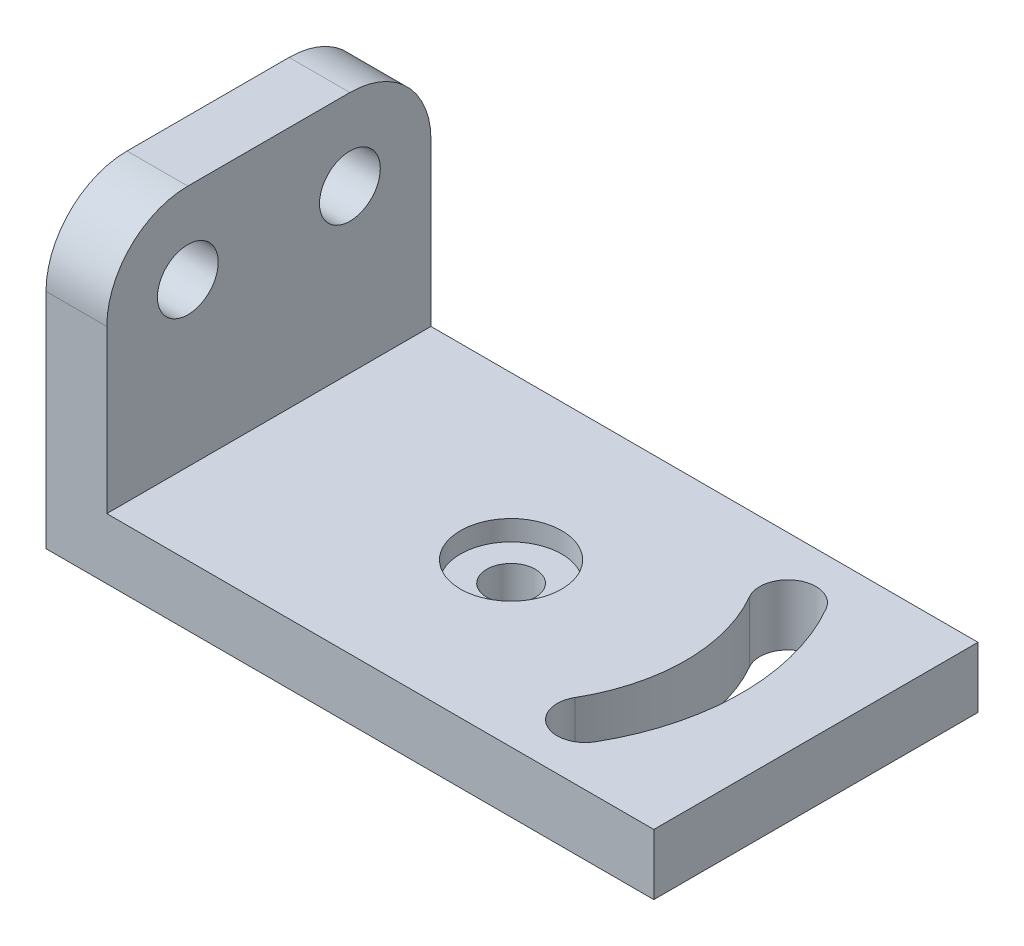
ISO-10303-21;
HEADER;
FILE_DESCRIPTION(('STEP AP214'),'2;1');
FILE_NAME('part.step','',(''),(''),'','','');
FILE_SCHEMA(('AUTOMOTIVE_DESIGN { 1 0 10303 214 1 1 1 1 }'));
ENDSEC;
DATA;
#1=APPLICATION_CONTEXT('core data for automotive mechanical design processes');
#2=APPLICATION_PROTOCOL_DEFINITION('international standard','automotive_design',2000,#1);
#3=PRODUCT_CONTEXT('',#1,'mechanical');
#4=PRODUCT('Part','Part','',(#3));
#5=PRODUCT_RELATED_PRODUCT_CATEGORY('part','',(#4));
#6=PRODUCT_DEFINITION_FORMATION('','',#4);
#7=PRODUCT_DEFINITION_CONTEXT('part definition',#1,'design');
#8=PRODUCT_DEFINITION('design','',#6,#7);
#9=PRODUCT_DEFINITION_SHAPE('','',#8);
#10=(LENGTH_UNIT() NAMED_UNIT(*) SI_UNIT(.MILLI.,.METRE.));
#11=(NAMED_UNIT(*) PLANE_ANGLE_UNIT() SI_UNIT($,.RADIAN.));
#12=(NAMED_UNIT(*) SI_UNIT($,.STERADIAN.) SOLID_ANGLE_UNIT());
#13=UNCERTAINTY_MEASURE_WITH_UNIT(LENGTH_MEASURE(1.E-05),#10,'distance_accuracy_value','');
#14=(GEOMETRIC_REPRESENTATION_CONTEXT(3) GLOBAL_UNCERTAINTY_ASSIGNED_CONTEXT((#13)) GLOBAL_UNIT_ASSIGNED_CONTEXT((#10,
#11,#12)) REPRESENTATION_CONTEXT('',''));
#15=CARTESIAN_POINT('',(0.,0.,0.));
#16=DIRECTION('',(0.,0.,1.));
#17=DIRECTION('',(1.,0.,0.));
#18=AXIS2_PLACEMENT_3D('',#15,#16,#17);
#19=CARTESIAN_POINT('',(0.,15.,40.));
#20=DIRECTION('',(0.,0.,1.));
#21=DIRECTION('',(1.,0.,0.));
#22=AXIS2_PLACEMENT_3D('',#19,#20,#21);
#23=PLANE('',#22);
#24=DIRECTION('',(0.,-1.,0.));
#25=VECTOR('',#24,1.);
#26=CARTESIAN_POINT('',(15.,75.,40.));
#27=LINE('',#26,#25);
#28=CARTESIAN_POINT('',(15.,55.,40.));
#29=VERTEX_POINT('',#28);
#30=CARTESIAN_POINT('',(15.,15.,40.));
#31=VERTEX_POINT('',#30);
#32=EDGE_CURVE('E138',#29,#31,#27,.T.);
#33=ORIENTED_EDGE('',*,*,#32,.F.);
#34=DIRECTION('',(1.,0.,0.));
#35=VECTOR('',#34,1.);
#36=CARTESIAN_POINT('',(0.,55.,40.));
#37=LINE('',#36,#35);
#38=CARTESIAN_POINT('',(0.,55.,40.));
#39=VERTEX_POINT('',#38);
#40=EDGE_CURVE('E11',#29,#39,#37,.F.);
#41=ORIENTED_EDGE('',*,*,#40,.T.);
#42=DIRECTION('',(0.,-1.,0.));
#43=VECTOR('',#42,1.);
#44=CARTESIAN_POINT('',(0.,15.,40.));
#45=LINE('',#44,#43);
#46=CARTESIAN_POINT('',(0.,0.,40.));
#47=VERTEX_POINT('',#46);
#48=EDGE_CURVE('E209',#39,#47,#45,.T.);
#49=ORIENTED_EDGE('',*,*,#48,.T.);
#50=DIRECTION('',(-1.,0.,0.));
#51=VECTOR('',#50,1.);
#52=CARTESIAN_POINT('',(0.,0.,40.));
#53=LINE('',#52,#51);
#54=CARTESIAN_POINT('',(150.,0.,40.));
#55=VERTEX_POINT('',#54);
#56=EDGE_CURVE('E198',#55,#47,#53,.T.);
#57=ORIENTED_EDGE('',*,*,#56,.F.);
#58=DIRECTION('',(0.,-1.,0.));
#59=VECTOR('',#58,1.);
#60=CARTESIAN_POINT('',(150.,15.,40.));
#61=LINE('',#60,#59);
#62=CARTESIAN_POINT('',(150.,15.,40.));
#63=VERTEX_POINT('',#62);
#64=EDGE_CURVE('E216',#63,#55,#61,.T.);
#65=ORIENTED_EDGE('',*,*,#64,.F.);
#66=DIRECTION('',(-1.,0.,0.));
#67=VECTOR('',#66,1.);
#68=CARTESIAN_POINT('',(0.,15.,40.));
#69=LINE('',#68,#67);
#70=EDGE_CURVE('E183',#63,#31,#69,.T.);
#71=ORIENTED_EDGE('',*,*,#70,.T.);
#72=EDGE_LOOP('',(#33,#41,#49,#57,#65,#71));
#73=FACE_BOUND('',#72,.T.);
#74=ADVANCED_FACE('F41',(#73),#23,.T.);
#75=CARTESIAN_POINT('',(150.,15.,0.));
#76=DIRECTION('',(1.,0.,0.));
#77=DIRECTION('',(0.,0.,-1.));
#78=AXIS2_PLACEMENT_3D('',#75,#76,#77);
#79=PLANE('',#78);
#80=DIRECTION('',(0.,0.,1.));
#81=VECTOR('',#80,1.);
#82=CARTESIAN_POINT('',(150.,0.,0.));
#83=LINE('',#82,#81);
#84=CARTESIAN_POINT('',(150.,0.,-40.));
#85=VERTEX_POINT('',#84);
#86=EDGE_CURVE('E203',#85,#55,#83,.T.);
#87=ORIENTED_EDGE('',*,*,#86,.F.);
#88=DIRECTION('',(0.,-1.,0.));
#89=VECTOR('',#88,1.);
#90=CARTESIAN_POINT('',(150.,15.,-40.));
#91=LINE('',#90,#89);
#92=CARTESIAN_POINT('',(150.,15.,-40.));
#93=VERTEX_POINT('',#92);
#94=EDGE_CURVE('E211',#93,#85,#91,.T.);
#95=ORIENTED_EDGE('',*,*,#94,.F.);
#96=DIRECTION('',(0.,0.,1.));
#97=VECTOR('',#96,1.);
#98=CARTESIAN_POINT('',(150.,15.,0.));
#99=LINE('',#98,#97);
#100=EDGE_CURVE('E149',#93,#63,#99,.T.);
#101=ORIENTED_EDGE('',*,*,#100,.T.);
#102=ORIENTED_EDGE('',*,*,#64,.T.);
#103=EDGE_LOOP('',(#87,#95,#101,#102));
#104=FACE_BOUND('',#103,.T.);
#105=ADVANCED_FACE('F283',(#104),#79,.T.);
#106=CARTESIAN_POINT('',(0.,15.,-40.));
#107=DIRECTION('',(0.,0.,-1.));
#108=DIRECTION('',(-1.,0.,0.));
#109=AXIS2_PLACEMENT_3D('',#106,#107,#108);
#110=PLANE('',#109);
#111=DIRECTION('',(0.,-1.,0.));
#112=VECTOR('',#111,1.);
#113=CARTESIAN_POINT('',(0.,15.,-40.));
#114=LINE('',#113,#112);
#115=CARTESIAN_POINT('',(0.,55.,-40.));
#116=VERTEX_POINT('',#115);
#117=CARTESIAN_POINT('',(0.,0.,-40.));
#118=VERTEX_POINT('',#117);
#119=EDGE_CURVE('E212',#116,#118,#114,.T.);
#120=ORIENTED_EDGE('',*,*,#119,.F.);
#121=DIRECTION('',(-1.,0.,0.));
#122=VECTOR('',#121,1.);
#123=CARTESIAN_POINT('',(0.,55.,-40.));
#124=LINE('',#123,#122);
#125=CARTESIAN_POINT('',(15.,55.,-40.));
#126=VERTEX_POINT('',#125);
#127=EDGE_CURVE('E66',#116,#126,#124,.F.);
#128=ORIENTED_EDGE('',*,*,#127,.T.);
#129=DIRECTION('',(0.,-1.,0.));
#130=VECTOR('',#129,1.);
#131=CARTESIAN_POINT('',(15.,75.,-40.));
#132=LINE('',#131,#130);
#133=CARTESIAN_POINT('',(15.,15.,-40.));
#134=VERTEX_POINT('',#133);
#135=EDGE_CURVE('E126',#126,#134,#132,.T.);
#136=ORIENTED_EDGE('',*,*,#135,.T.);
#137=DIRECTION('',(1.,0.,0.));
#138=VECTOR('',#137,1.);
#139=CARTESIAN_POINT('',(0.,15.,-40.));
#140=LINE('',#139,#138);
#141=EDGE_CURVE('E135',#134,#93,#140,.T.);
#142=ORIENTED_EDGE('',*,*,#141,.T.);
#143=ORIENTED_EDGE('',*,*,#94,.T.);
#144=DIRECTION('',(1.,0.,0.));
#145=VECTOR('',#144,1.);
#146=CARTESIAN_POINT('',(0.,0.,-40.));
#147=LINE('',#146,#145);
#148=EDGE_CURVE('E202',#118,#85,#147,.T.);
#149=ORIENTED_EDGE('',*,*,#148,.F.);
#150=EDGE_LOOP('',(#120,#128,#136,#142,#143,#149));
#151=FACE_BOUND('',#150,.T.);
#152=ADVANCED_FACE('F131',(#151),#110,.T.);
#153=CARTESIAN_POINT('',(118.069662559794,15.,-25.0000000000001));
#154=DIRECTION('',(0.,-1.,0.));
#155=DIRECTION('',(0.,0.,-1.));
#156=AXIS2_PLACEMENT_3D('',#153,#154,#155);
#157=CYLINDRICAL_SURFACE('',#156,6.92452153915603);
#158=CARTESIAN_POINT('',(118.069662559794,0.,-25.0000000000001));
#159=DIRECTION('',(0.,1.,0.));
#160=DIRECTION('',(0.,0.,1.));
#161=AXIS2_PLACEMENT_3D('',#158,#159,#160);
#162=CIRCLE('',#161,6.92452153915603);
#163=CARTESIAN_POINT('',(124.066474121756,0.,-28.4622607695782));
#164=VERTEX_POINT('',#163);
#165=CARTESIAN_POINT('',(112.072850997832,0.,-21.5377392304221));
#166=VERTEX_POINT('',#165);
#167=EDGE_CURVE('E168',#164,#166,#162,.T.);
#168=ORIENTED_EDGE('',*,*,#167,.F.);
#169=DIRECTION('',(0.,-1.,0.));
#170=VECTOR('',#169,1.);
#171=CARTESIAN_POINT('',(124.066474121756,15.,-28.4622607695782));
#172=LINE('',#171,#170);
#173=CARTESIAN_POINT('',(124.066474121756,15.,-28.4622607695782));
#174=VERTEX_POINT('',#173);
#175=EDGE_CURVE('E215',#174,#164,#172,.T.);
#176=ORIENTED_EDGE('',*,*,#175,.F.);
#177=CARTESIAN_POINT('',(118.069662559794,15.,-25.0000000000001));
#178=DIRECTION('',(0.,1.,0.));
#179=DIRECTION('',(0.,0.,1.));
#180=AXIS2_PLACEMENT_3D('',#177,#178,#179);
#181=CIRCLE('',#180,6.92452153915603);
#182=CARTESIAN_POINT('',(112.072850997832,15.,-21.5377392304221));
#183=VERTEX_POINT('',#182);
#184=EDGE_CURVE('E169',#174,#183,#181,.T.);
#185=ORIENTED_EDGE('',*,*,#184,.T.);
#186=DIRECTION('',(0.,-1.,0.));
#187=VECTOR('',#186,1.);
#188=CARTESIAN_POINT('',(112.072850997832,15.,-21.5377392304221));
#189=LINE('',#188,#187);
#190=EDGE_CURVE('E146',#183,#166,#189,.T.);
#191=ORIENTED_EDGE('',*,*,#190,.T.);
#192=EDGE_LOOP('',(#168,#176,#185,#191));
#193=FACE_BOUND('',#192,.T.);
#194=ADVANCED_FACE('F317',(#193),#157,.F.);
#195=CARTESIAN_POINT('',(74.7683923705722,15.,0.));
#196=DIRECTION('',(0.,-1.,0.));
#197=DIRECTION('',(0.,0.,-1.));
#198=AXIS2_PLACEMENT_3D('',#195,#196,#197);
#199=CYLINDRICAL_SURFACE('',#198,56.924521539156);
#200=CARTESIAN_POINT('',(74.7683923705722,0.,0.));
#201=DIRECTION('',(0.,1.,0.));
#202=DIRECTION('',(0.,0.,1.));
#203=AXIS2_PLACEMENT_3D('',#200,#201,#202);
#204=CIRCLE('',#203,56.924521539156);
#205=CARTESIAN_POINT('',(124.066474121756,0.,28.4622607695781));
#206=VERTEX_POINT('',#205);
#207=EDGE_CURVE('E186',#206,#164,#204,.T.);
#208=ORIENTED_EDGE('',*,*,#207,.F.);
#209=DIRECTION('',(0.,-1.,0.));
#210=VECTOR('',#209,1.);
#211=CARTESIAN_POINT('',(124.066474121756,15.,28.4622607695781));
#212=LINE('',#211,#210);
#213=CARTESIAN_POINT('',(124.066474121756,15.,28.4622607695781));
#214=VERTEX_POINT('',#213);
#215=EDGE_CURVE('E225',#214,#206,#212,.T.);
#216=ORIENTED_EDGE('',*,*,#215,.F.);
#217=CARTESIAN_POINT('',(74.7683923705722,15.,0.));
#218=DIRECTION('',(0.,1.,0.));
#219=DIRECTION('',(0.,0.,1.));
#220=AXIS2_PLACEMENT_3D('',#217,#218,#219);
#221=CIRCLE('',#220,56.924521539156);
#222=EDGE_CURVE('E175',#214,#174,#221,.T.);
#223=ORIENTED_EDGE('',*,*,#222,.T.);
#224=ORIENTED_EDGE('',*,*,#175,.T.);
#225=EDGE_LOOP('',(#208,#216,#223,#224));
#226=FACE_BOUND('',#225,.T.);
#227=ADVANCED_FACE('F312',(#226),#199,.F.);
#228=CARTESIAN_POINT('',(118.069662559794,15.,25.0000000000001));
#229=DIRECTION('',(0.,-1.,0.));
#230=DIRECTION('',(0.,0.,-1.));
#231=AXIS2_PLACEMENT_3D('',#228,#229,#230);
#232=CYLINDRICAL_SURFACE('',#231,6.92452153915602);
#233=CARTESIAN_POINT('',(118.069662559794,0.,25.0000000000001));
#234=DIRECTION('',(0.,1.,0.));
#235=DIRECTION('',(0.,0.,1.));
#236=AXIS2_PLACEMENT_3D('',#233,#234,#235);
#237=CIRCLE('',#236,6.92452153915602);
#238=CARTESIAN_POINT('',(112.072850997833,0.,21.537739230422));
#239=VERTEX_POINT('',#238);
#240=EDGE_CURVE('E195',#239,#206,#237,.T.);
#241=ORIENTED_EDGE('',*,*,#240,.F.);
#242=DIRECTION('',(0.,-1.,0.));
#243=VECTOR('',#242,1.);
#244=CARTESIAN_POINT('',(112.072850997833,15.,21.537739230422));
#245=LINE('',#244,#243);
#246=CARTESIAN_POINT('',(112.072850997833,15.,21.537739230422));
#247=VERTEX_POINT('',#246);
#248=EDGE_CURVE('E219',#247,#239,#245,.T.);
#249=ORIENTED_EDGE('',*,*,#248,.F.);
#250=CARTESIAN_POINT('',(118.069662559794,15.,25.0000000000001));
#251=DIRECTION('',(0.,1.,0.));
#252=DIRECTION('',(0.,0.,1.));
#253=AXIS2_PLACEMENT_3D('',#250,#251,#252);
#254=CIRCLE('',#253,6.92452153915602);
#255=EDGE_CURVE('E176',#247,#214,#254,.T.);
#256=ORIENTED_EDGE('',*,*,#255,.T.);
#257=ORIENTED_EDGE('',*,*,#215,.T.);
#258=EDGE_LOOP('',(#241,#249,#256,#257));
#259=FACE_BOUND('',#258,.T.);
#260=ADVANCED_FACE('F306',(#259),#232,.F.);
#261=CARTESIAN_POINT('',(74.7683923705722,15.,0.));
#262=DIRECTION('',(0.,-1.,0.));
#263=DIRECTION('',(0.,0.,-1.));
#264=AXIS2_PLACEMENT_3D('',#261,#262,#263);
#265=CYLINDRICAL_SURFACE('',#264,12.5);
#266=CARTESIAN_POINT('',(74.7683923705722,10.,0.));
#267=DIRECTION('',(0.,1.,0.));
#268=DIRECTION('',(0.,0.,1.));
#269=AXIS2_PLACEMENT_3D('',#266,#267,#268);
#270=CIRCLE('',#269,12.5);
#271=CARTESIAN_POINT('',(74.7683923705722,10.,12.5));
#272=VERTEX_POINT('',#271);
#273=EDGE_CURVE('E218',#272,#272,#270,.T.);
#274=ORIENTED_EDGE('',*,*,#273,.F.);
#275=EDGE_LOOP('',(#274));
#276=FACE_BOUND('',#275,.T.);
#277=CARTESIAN_POINT('',(74.7683923705722,15.,0.));
#278=DIRECTION('',(0.,1.,0.));
#279=DIRECTION('',(0.,0.,1.));
#280=AXIS2_PLACEMENT_3D('',#277,#278,#279);
#281=CIRCLE('',#280,12.5);
#282=CARTESIAN_POINT('',(74.7683923705722,15.,12.5));
#283=VERTEX_POINT('',#282);
#284=EDGE_CURVE('E181',#283,#283,#281,.T.);
#285=ORIENTED_EDGE('',*,*,#284,.T.);
#286=EDGE_LOOP('',(#285));
#287=FACE_BOUND('',#286,.T.);
#288=ADVANCED_FACE('F303',(#276,#287),#265,.F.);
#289=CARTESIAN_POINT('',(74.7683923705722,15.,0.));
#290=DIRECTION('',(0.,-1.,0.));
#291=DIRECTION('',(0.,0.,-1.));
#292=AXIS2_PLACEMENT_3D('',#289,#290,#291);
#293=CYLINDRICAL_SURFACE('',#292,43.075478460844);
#294=CARTESIAN_POINT('',(74.7683923705722,0.,0.));
#295=DIRECTION('',(0.,1.,0.));
#296=DIRECTION('',(0.,0.,1.));
#297=AXIS2_PLACEMENT_3D('',#294,#295,#296);
#298=CIRCLE('',#297,43.075478460844);
#299=EDGE_CURVE('E193',#239,#166,#298,.T.);
#300=ORIENTED_EDGE('',*,*,#299,.T.);
#301=ORIENTED_EDGE('',*,*,#190,.F.);
#302=CARTESIAN_POINT('',(74.7683923705722,15.,0.));
#303=DIRECTION('',(0.,1.,0.));
#304=DIRECTION('',(0.,0.,1.));
#305=AXIS2_PLACEMENT_3D('',#302,#303,#304);
#306=CIRCLE('',#305,43.075478460844);
#307=EDGE_CURVE('E177',#247,#183,#306,.T.);
#308=ORIENTED_EDGE('',*,*,#307,.F.);
#309=ORIENTED_EDGE('',*,*,#248,.T.);
#310=EDGE_LOOP('',(#300,#301,#308,#309));
#311=FACE_BOUND('',#310,.T.);
#312=ADVANCED_FACE('F261',(#311),#293,.T.);
#313=CARTESIAN_POINT('',(0.,15.,0.));
#314=DIRECTION('',(1.,0.,0.));
#315=DIRECTION('',(0.,0.,-1.));
#316=AXIS2_PLACEMENT_3D('',#313,#314,#315);
#317=PLANE('',#316);
#318=CARTESIAN_POINT('',(0.,55.,-20.));
#319=DIRECTION('',(1.,0.,0.));
#320=DIRECTION('',(0.,0.,-1.));
#321=AXIS2_PLACEMENT_3D('',#318,#319,#320);
#322=CIRCLE('',#321,7.5);
#323=CARTESIAN_POINT('',(0.,55.,-27.5));
#324=VERTEX_POINT('',#323);
#325=EDGE_CURVE('E153',#324,#324,#322,.T.);
#326=ORIENTED_EDGE('',*,*,#325,.T.);
#327=EDGE_LOOP('',(#326));
#328=FACE_BOUND('',#327,.T.);
#329=CARTESIAN_POINT('',(0.,55.,20.));
#330=DIRECTION('',(1.,0.,0.));
#331=DIRECTION('',(0.,0.,-1.));
#332=AXIS2_PLACEMENT_3D('',#329,#330,#331);
#333=CIRCLE('',#332,7.5);
#334=CARTESIAN_POINT('',(0.,55.,12.5));
#335=VERTEX_POINT('',#334);
#336=EDGE_CURVE('E241',#335,#335,#333,.T.);
#337=ORIENTED_EDGE('',*,*,#336,.T.);
#338=EDGE_LOOP('',(#337));
#339=FACE_BOUND('',#338,.T.);
#340=DIRECTION('',(0.,0.,1.));
#341=VECTOR('',#340,1.);
#342=CARTESIAN_POINT('',(0.,75.,-40.));
#343=LINE('',#342,#341);
#344=CARTESIAN_POINT('',(0.,75.,-20.));
#345=VERTEX_POINT('',#344);
#346=CARTESIAN_POINT('',(0.,75.,20.));
#347=VERTEX_POINT('',#346);
#348=EDGE_CURVE('E155',#345,#347,#343,.T.);
#349=ORIENTED_EDGE('',*,*,#348,.F.);
#350=CARTESIAN_POINT('',(0.,55.,-20.));
#351=DIRECTION('',(1.,0.,0.));
#352=DIRECTION('',(0.,0.,-1.));
#353=AXIS2_PLACEMENT_3D('',#350,#351,#352);
#354=CIRCLE('',#353,20.);
#355=EDGE_CURVE('E232',#345,#116,#354,.F.);
#356=ORIENTED_EDGE('',*,*,#355,.T.);
#357=ORIENTED_EDGE('',*,*,#119,.T.);
#358=DIRECTION('',(0.,0.,1.));
#359=VECTOR('',#358,1.);
#360=CARTESIAN_POINT('',(0.,0.,0.));
#361=LINE('',#360,#359);
#362=EDGE_CURVE('E173',#118,#47,#361,.T.);
#363=ORIENTED_EDGE('',*,*,#362,.T.);
#364=ORIENTED_EDGE('',*,*,#48,.F.);
#365=CARTESIAN_POINT('',(0.,55.,20.));
#366=DIRECTION('',(1.,0.,0.));
#367=DIRECTION('',(0.,0.,-1.));
#368=AXIS2_PLACEMENT_3D('',#365,#366,#367);
#369=CIRCLE('',#368,20.);
#370=EDGE_CURVE('E231',#39,#347,#369,.F.);
#371=ORIENTED_EDGE('',*,*,#370,.T.);
#372=EDGE_LOOP('',(#349,#356,#357,#363,#364,#371));
#373=FACE_BOUND('',#372,.T.);
#374=ADVANCED_FACE('F256',(#328,#339,#373),#317,.F.);
#375=CARTESIAN_POINT('',(0.,15.,0.));
#376=DIRECTION('',(0.,1.,0.));
#377=DIRECTION('',(0.,0.,1.));
#378=AXIS2_PLACEMENT_3D('',#375,#376,#377);
#379=PLANE('',#378);
#380=DIRECTION('',(0.,0.,-1.));
#381=VECTOR('',#380,1.);
#382=CARTESIAN_POINT('',(15.,15.,-40.));
#383=LINE('',#382,#381);
#384=EDGE_CURVE('E143',#31,#134,#383,.T.);
#385=ORIENTED_EDGE('',*,*,#384,.F.);
#386=ORIENTED_EDGE('',*,*,#70,.F.);
#387=ORIENTED_EDGE('',*,*,#100,.F.);
#388=ORIENTED_EDGE('',*,*,#141,.F.);
#389=EDGE_LOOP('',(#385,#386,#387,#388));
#390=FACE_BOUND('',#389,.T.);
#391=ORIENTED_EDGE('',*,*,#184,.F.);
#392=ORIENTED_EDGE('',*,*,#222,.F.);
#393=ORIENTED_EDGE('',*,*,#255,.F.);
#394=ORIENTED_EDGE('',*,*,#307,.T.);
#395=EDGE_LOOP('',(#391,#392,#393,#394));
#396=FACE_BOUND('',#395,.T.);
#397=ORIENTED_EDGE('',*,*,#284,.F.);
#398=EDGE_LOOP('',(#397));
#399=FACE_BOUND('',#398,.T.);
#400=ADVANCED_FACE('F145',(#390,#396,#399),#379,.T.);
#401=CARTESIAN_POINT('',(0.,0.,0.));
#402=DIRECTION('',(0.,1.,0.));
#403=DIRECTION('',(0.,0.,1.));
#404=AXIS2_PLACEMENT_3D('',#401,#402,#403);
#405=PLANE('',#404);
#406=ORIENTED_EDGE('',*,*,#167,.T.);
#407=ORIENTED_EDGE('',*,*,#299,.F.);
#408=ORIENTED_EDGE('',*,*,#240,.T.);
#409=ORIENTED_EDGE('',*,*,#207,.T.);
#410=EDGE_LOOP('',(#406,#407,#408,#409));
#411=FACE_BOUND('',#410,.T.);
#412=ORIENTED_EDGE('',*,*,#56,.T.);
#413=ORIENTED_EDGE('',*,*,#362,.F.);
#414=ORIENTED_EDGE('',*,*,#148,.T.);
#415=ORIENTED_EDGE('',*,*,#86,.T.);
#416=EDGE_LOOP('',(#412,#413,#414,#415));
#417=FACE_BOUND('',#416,.T.);
#418=CARTESIAN_POINT('',(74.7683923705722,0.,0.));
#419=DIRECTION('',(0.,1.,0.));
#420=DIRECTION('',(0.,0.,1.));
#421=AXIS2_PLACEMENT_3D('',#418,#419,#420);
#422=CIRCLE('',#421,6.00000000000001);
#423=CARTESIAN_POINT('',(74.7683923705722,0.,6.00000000000001));
#424=VERTEX_POINT('',#423);
#425=EDGE_CURVE('E162',#424,#424,#422,.T.);
#426=ORIENTED_EDGE('',*,*,#425,.T.);
#427=EDGE_LOOP('',(#426));
#428=FACE_BOUND('',#427,.T.);
#429=ADVANCED_FACE('F276',(#411,#417,#428),#405,.F.);
#430=CARTESIAN_POINT('',(74.7683923705722,10.,0.));
#431=DIRECTION('',(0.,-1.,0.));
#432=DIRECTION('',(0.,0.,-1.));
#433=AXIS2_PLACEMENT_3D('',#430,#431,#432);
#434=CYLINDRICAL_SURFACE('',#433,6.00000000000001);
#435=CARTESIAN_POINT('',(74.7683923705722,10.,0.));
#436=DIRECTION('',(0.,1.,0.));
#437=DIRECTION('',(0.,0.,1.));
#438=AXIS2_PLACEMENT_3D('',#435,#436,#437);
#439=CIRCLE('',#438,6.00000000000001);
#440=CARTESIAN_POINT('',(74.7683923705722,10.,6.00000000000001));
#441=VERTEX_POINT('',#440);
#442=EDGE_CURVE('E161',#441,#441,#439,.T.);
#443=ORIENTED_EDGE('',*,*,#442,.T.);
#444=EDGE_LOOP('',(#443));
#445=FACE_BOUND('',#444,.T.);
#446=ORIENTED_EDGE('',*,*,#425,.F.);
#447=EDGE_LOOP('',(#446));
#448=FACE_BOUND('',#447,.T.);
#449=ADVANCED_FACE('F338',(#445,#448),#434,.F.);
#450=CARTESIAN_POINT('',(0.,10.,0.));
#451=DIRECTION('',(0.,1.,0.));
#452=DIRECTION('',(0.,0.,1.));
#453=AXIS2_PLACEMENT_3D('',#450,#451,#452);
#454=PLANE('',#453);
#455=ORIENTED_EDGE('',*,*,#442,.F.);
#456=EDGE_LOOP('',(#455));
#457=FACE_BOUND('',#456,.T.);
#458=ORIENTED_EDGE('',*,*,#273,.T.);
#459=EDGE_LOOP('',(#458));
#460=FACE_BOUND('',#459,.T.);
#461=ADVANCED_FACE('F343',(#457,#460),#454,.T.);
#462=CARTESIAN_POINT('',(15.,75.,-40.));
#463=DIRECTION('',(-1.,0.,0.));
#464=DIRECTION('',(0.,0.,1.));
#465=AXIS2_PLACEMENT_3D('',#462,#463,#464);
#466=PLANE('',#465);
#467=CARTESIAN_POINT('',(15.,55.,-20.));
#468=DIRECTION('',(-1.,0.,0.));
#469=DIRECTION('',(0.,0.,1.));
#470=AXIS2_PLACEMENT_3D('',#467,#468,#469);
#471=CIRCLE('',#470,7.5);
#472=CARTESIAN_POINT('',(15.,55.,-12.5));
#473=VERTEX_POINT('',#472);
#474=EDGE_CURVE('E44',#473,#473,#471,.T.);
#475=ORIENTED_EDGE('',*,*,#474,.T.);
#476=EDGE_LOOP('',(#475));
#477=FACE_BOUND('',#476,.T.);
#478=CARTESIAN_POINT('',(15.,55.,20.));
#479=DIRECTION('',(-1.,0.,0.));
#480=DIRECTION('',(0.,0.,1.));
#481=AXIS2_PLACEMENT_3D('',#478,#479,#480);
#482=CIRCLE('',#481,7.5);
#483=CARTESIAN_POINT('',(15.,55.,27.5));
#484=VERTEX_POINT('',#483);
#485=EDGE_CURVE('E237',#484,#484,#482,.T.);
#486=ORIENTED_EDGE('',*,*,#485,.T.);
#487=EDGE_LOOP('',(#486));
#488=FACE_BOUND('',#487,.T.);
#489=ORIENTED_EDGE('',*,*,#135,.F.);
#490=CARTESIAN_POINT('',(15.,55.,-20.));
#491=DIRECTION('',(-1.,0.,0.));
#492=DIRECTION('',(0.,0.,1.));
#493=AXIS2_PLACEMENT_3D('',#490,#491,#492);
#494=CIRCLE('',#493,20.);
#495=CARTESIAN_POINT('',(15.,75.,-20.));
#496=VERTEX_POINT('',#495);
#497=EDGE_CURVE('E49',#126,#496,#494,.F.);
#498=ORIENTED_EDGE('',*,*,#497,.T.);
#499=DIRECTION('',(0.,0.,-1.));
#500=VECTOR('',#499,1.);
#501=CARTESIAN_POINT('',(15.,75.,-40.));
#502=LINE('',#501,#500);
#503=CARTESIAN_POINT('',(15.,75.,20.));
#504=VERTEX_POINT('',#503);
#505=EDGE_CURVE('E140',#504,#496,#502,.T.);
#506=ORIENTED_EDGE('',*,*,#505,.F.);
#507=CARTESIAN_POINT('',(15.,55.,20.));
#508=DIRECTION('',(-1.,0.,0.));
#509=DIRECTION('',(0.,0.,1.));
#510=AXIS2_PLACEMENT_3D('',#507,#508,#509);
#511=CIRCLE('',#510,20.);
#512=EDGE_CURVE('E59',#504,#29,#511,.F.);
#513=ORIENTED_EDGE('',*,*,#512,.T.);
#514=ORIENTED_EDGE('',*,*,#32,.T.);
#515=ORIENTED_EDGE('',*,*,#384,.T.);
#516=EDGE_LOOP('',(#489,#498,#506,#513,#514,#515));
#517=FACE_BOUND('',#516,.T.);
#518=ADVANCED_FACE('F151',(#477,#488,#517),#466,.F.);
#519=CARTESIAN_POINT('',(0.,75.,0.));
#520=DIRECTION('',(0.,1.,0.));
#521=DIRECTION('',(0.,0.,1.));
#522=AXIS2_PLACEMENT_3D('',#519,#520,#521);
#523=PLANE('',#522);
#524=ORIENTED_EDGE('',*,*,#505,.T.);
#525=DIRECTION('',(-1.,0.,0.));
#526=VECTOR('',#525,1.);
#527=CARTESIAN_POINT('',(0.,75.,-20.));
#528=LINE('',#527,#526);
#529=EDGE_CURVE('E229',#496,#345,#528,.T.);
#530=ORIENTED_EDGE('',*,*,#529,.T.);
#531=ORIENTED_EDGE('',*,*,#348,.T.);
#532=DIRECTION('',(1.,0.,0.));
#533=VECTOR('',#532,1.);
#534=CARTESIAN_POINT('',(0.,75.,20.));
#535=LINE('',#534,#533);
#536=EDGE_CURVE('E227',#347,#504,#535,.T.);
#537=ORIENTED_EDGE('',*,*,#536,.T.);
#538=EDGE_LOOP('',(#524,#530,#531,#537));
#539=FACE_BOUND('',#538,.T.);
#540=ADVANCED_FACE('F269',(#539),#523,.T.);
#541=CARTESIAN_POINT('',(0.,55.,-20.));
#542=DIRECTION('',(-1.,0.,0.));
#543=DIRECTION('',(0.,0.,1.));
#544=AXIS2_PLACEMENT_3D('',#541,#542,#543);
#545=CYLINDRICAL_SURFACE('',#544,20.);
#546=ORIENTED_EDGE('',*,*,#497,.F.);
#547=ORIENTED_EDGE('',*,*,#127,.F.);
#548=ORIENTED_EDGE('',*,*,#355,.F.);
#549=ORIENTED_EDGE('',*,*,#529,.F.);
#550=EDGE_LOOP('',(#546,#547,#548,#549));
#551=FACE_BOUND('',#550,.T.);
#552=ADVANCED_FACE('F284',(#551),#545,.T.);
#553=CARTESIAN_POINT('',(0.,55.,20.));
#554=DIRECTION('',(1.,0.,0.));
#555=DIRECTION('',(0.,0.,-1.));
#556=AXIS2_PLACEMENT_3D('',#553,#554,#555);
#557=CYLINDRICAL_SURFACE('',#556,20.);
#558=ORIENTED_EDGE('',*,*,#370,.F.);
#559=ORIENTED_EDGE('',*,*,#40,.F.);
#560=ORIENTED_EDGE('',*,*,#512,.F.);
#561=ORIENTED_EDGE('',*,*,#536,.F.);
#562=EDGE_LOOP('',(#558,#559,#560,#561));
#563=FACE_BOUND('',#562,.T.);
#564=ADVANCED_FACE('F43',(#563),#557,.T.);
#565=CARTESIAN_POINT('',(-25.,55.,20.));
#566=DIRECTION('',(1.,0.,0.));
#567=DIRECTION('',(0.,0.,-1.));
#568=AXIS2_PLACEMENT_3D('',#565,#566,#567);
#569=CYLINDRICAL_SURFACE('',#568,7.5);
#570=ORIENTED_EDGE('',*,*,#485,.F.);
#571=EDGE_LOOP('',(#570));
#572=FACE_BOUND('',#571,.T.);
#573=ORIENTED_EDGE('',*,*,#336,.F.);
#574=EDGE_LOOP('',(#573));
#575=FACE_BOUND('',#574,.T.);
#576=ADVANCED_FACE('F253',(#572,#575),#569,.F.);
#577=CARTESIAN_POINT('',(-25.,55.,-20.));
#578=DIRECTION('',(1.,0.,0.));
#579=DIRECTION('',(0.,0.,-1.));
#580=AXIS2_PLACEMENT_3D('',#577,#578,#579);
#581=CYLINDRICAL_SURFACE('',#580,7.5);
#582=ORIENTED_EDGE('',*,*,#474,.F.);
#583=EDGE_LOOP('',(#582));
#584=FACE_BOUND('',#583,.T.);
#585=ORIENTED_EDGE('',*,*,#325,.F.);
#586=EDGE_LOOP('',(#585));
#587=FACE_BOUND('',#586,.T.);
#588=ADVANCED_FACE('F255',(#584,#587),#581,.F.);
#589=CLOSED_SHELL('',(#74,#105,#152,#194,#227,#260,#288,#312,#374,#400,#429,#449,#461,#518,#540,
#552,#564,#576,#588));
#590=MANIFOLD_SOLID_BREP('B2',#589);
#591=ADVANCED_BREP_SHAPE_REPRESENTATION('',(#18,#590),#14);
#592=SHAPE_DEFINITION_REPRESENTATION(#9,#591);
ENDSEC;
END-ISO-10303-21;
